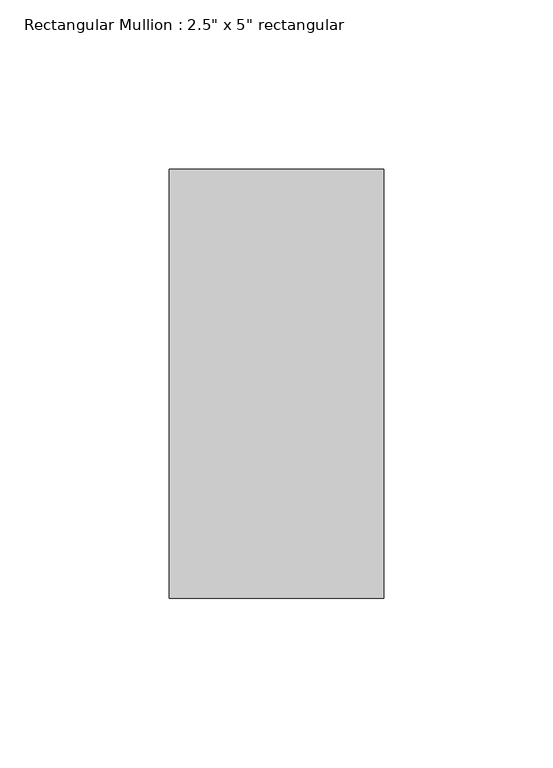
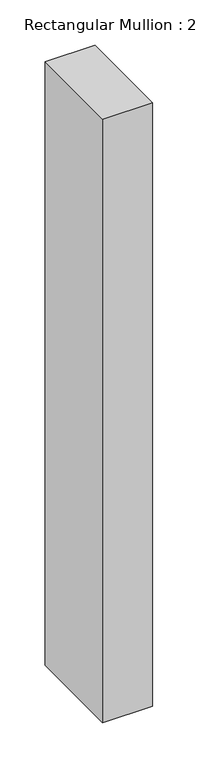
"""IFC4 building model written with IfcOpenShell, lengths in millimetres: member geometry."""

from ifc_helpers import new_model, si_unit, frame, origin, place, context, project, spatial, polyline, outline, extrude, source, transform, mapped, element, save


def member_8b3492ed(model_context):
    return source(origin(), model_context, "Body", "SweptSolid", [
        extrude(outline(polyline([(0.0, 63.5), (0.0, -63.5), (-63.5, -63.5), (-63.5, 63.5), (0.0, 63.5)])), frame((0.0, 0.0, -812.8), z_axis=(0.0, 0.0, 1.0), x_axis=(1.0, 0.0, 0.0)), (0.0, 0.0, 1.0), 812.8),
    ])


if __name__ == "__main__":
    model = new_model("IFC4")
    model_context = context("Model", 3, world=origin())
    ifc_project = project(units=[si_unit("LENGTHUNIT", "METRE", prefix="MILLI")], contexts=[model_context])
    site = spatial("IfcSite", under=ifc_project)
    building = spatial("IfcBuilding", under=site)
    placement = place(None, origin())
    member_shape = member_8b3492ed(model_context)
    element("IfcMember", 1, ObjectType="Rectangular Mullion : 2.5\" x 5\" rectangular", at=placement, inside=building, context=model_context, shape_type="MappedRepresentation", body=[
        mapped(member_shape, transform((0.0, 0.0, 0.0), x_axis=(1.0, 0.0, 0.0), y_axis=(0.0, 1.0, 0.0), z_axis=(0.0, 0.0, 1.0))),
    ])
    save(model, "model.ifc")

# Revit data of these elements
# Type "Rectangular Mullion : 2.5\" x 5\" rectangular"
#   built-in parameter 1007304 = 0.416667 (stored number, unit not read)
#   built-in parameter 1007301 = 0.104167 (stored number, unit not read)
#   built-in parameter 1007300 = 0.104167 (stored number, unit not read)
